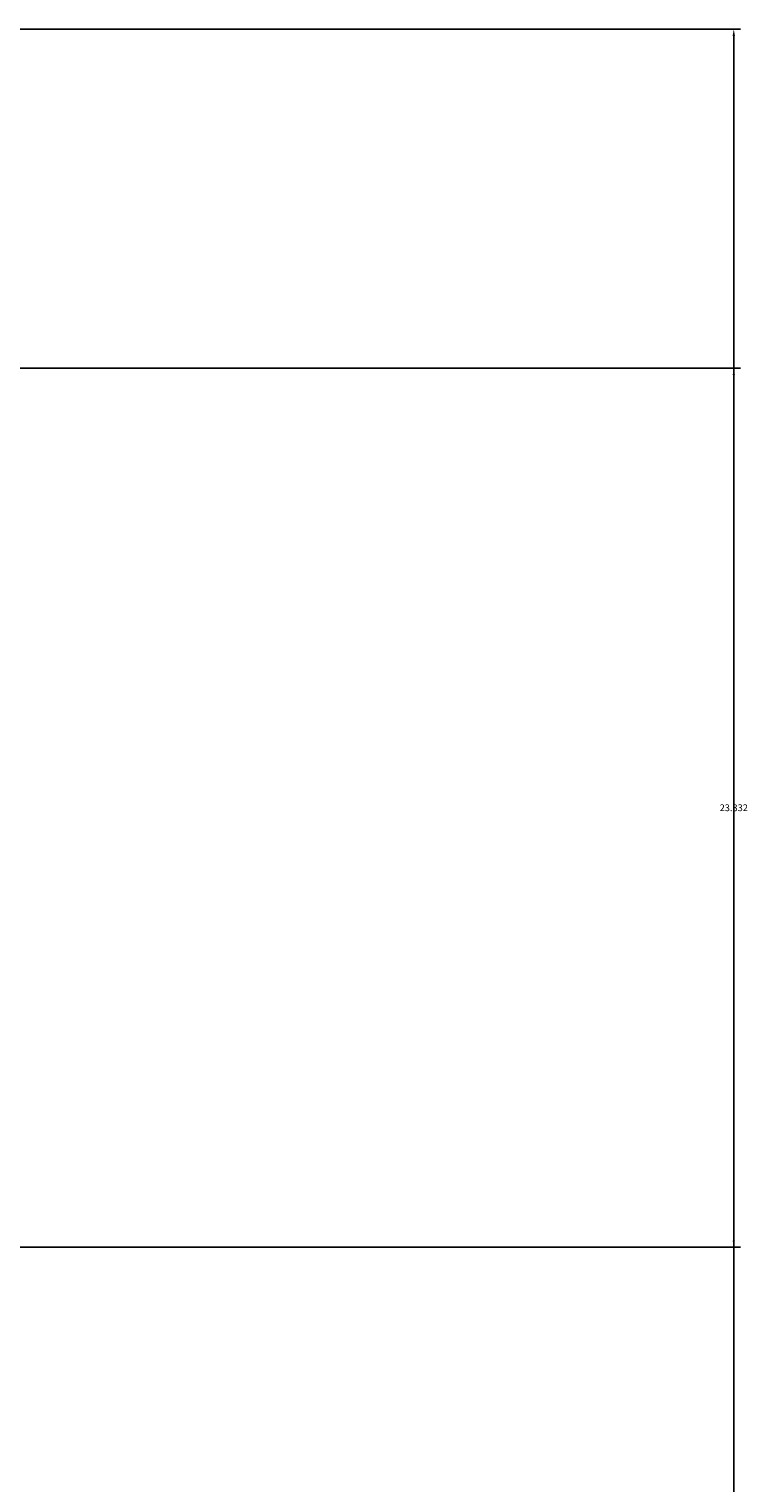
# Model space of a CAD drawing. Units: inches. Extents: x 2307 to 2544, y 2171 to 2540.
# Tile 51 of 52: x 2525 to 2544, y 2482 to 2521. Entities that reach past the tile are written whole.
import ezdxf

# ---------------------------------------------------------------- set-up
doc = ezdxf.new("R2010")
doc.units = ezdxf.units.IN
doc.layers.add('A-ANNO-DIMS', color=2, linetype='Continuous', lineweight=18)
doc.styles.get("Standard").update_dxf_attribs({"font": 'arial.ttf'})
doc.dimstyles.get("Standard").update_dxf_attribs({"dimtxt": 0.18, "dimasz": 0.18, "dimexe": 0.18, "dimexo": 0.0625, "dimgap": 0.09, "dimtad": 0, "dimtih": 1, "dimtoh": 1, "dimdec": 4, "dimzin": 0, "dimdsep": 46, "dimtxsty": 'Standard', "dimcen": 0.09, "dimadec": 0, "dimazin": 0, "dimtfac": 1, "dimtdec": 4, "dimtofl": 0, "dimtmove": 0, "dimatfit": 3, "dimfxl": 1, "dimtolj": 1, "dimtzin": 0, "dimarcsym": 0})

# ---------------------------------------------------------------- blocks, each defined once
blk = doc.blocks.new('*D37')
at = {"layer": 'A-ANNO-DIMS', "color": 0, "lineweight": -2, "transparency": 16777216}
for p, q in [((2524.758, 2520.51), (2544.026, 2520.51)), ((2543.846, 2520.33), (2543.846, 2355.692)), ((2543.846, 2190.69), (2543.846, 2355.328)), ((2524.758, 2190.51), (2544.026, 2190.51))]:
    blk.add_line(p, q, dxfattribs=at)
at = {"layer": 'A-ANNO-DIMS', "color": 0, "transparency": 16777216}
for points in [[(2543.816, 2520.33), (2543.876, 2520.33), (2543.846, 2520.51)], [(2543.816, 2190.69), (2543.876, 2190.69), (2543.846, 2190.51)]]:
    blk.add_solid(points, dxfattribs=at)
at = {"layer": 'Defpoints', "color": 0, "transparency": 16777216}
for p in [(2524.696, 2520.51), (2543.846, 2520.51), (2524.696, 2190.51)]:
    blk.add_point(p, dxfattribs=at)
at = {"layer": 'A-ANNO-DIMS', "color": 0, "transparency": 16777216, "insert": (2543.846, 2355.51), "char_height": 0.18, "attachment_point": 5}
blk.add_mtext('\\A1;330', dxfattribs=at)
blk = doc.blocks.new('*D64')
at = {"layer": 'A-ANNO-DIMS', "color": 0, "lineweight": -2, "transparency": 16777216}
for p, q in [((2515.758, 2511.51), (2544.026, 2511.51)), ((2543.846, 2511.33), (2543.846, 2500.025)), ((2543.846, 2488.357), (2543.846, 2499.661)), ((2514.64, 2488.177), (2544.026, 2488.177))]:
    blk.add_line(p, q, dxfattribs=at)
at = {"layer": 'A-ANNO-DIMS', "color": 0, "transparency": 16777216}
for points in [[(2543.816, 2511.33), (2543.876, 2511.33), (2543.846, 2511.51)], [(2543.816, 2488.357), (2543.876, 2488.357), (2543.846, 2488.177)]]:
    blk.add_solid(points, dxfattribs=at)
at = {"layer": 'Defpoints', "color": 0, "transparency": 16777216}
for p in [(2515.696, 2511.51), (2514.578, 2488.177), (2543.846, 2488.177)]:
    blk.add_point(p, dxfattribs=at)
at = {"layer": 'A-ANNO-DIMS', "color": 0, "transparency": 16777216, "insert": (2543.846, 2499.843), "char_height": 0.18, "attachment_point": 5}
blk.add_mtext('\\A1;23.332', dxfattribs=at)

msp = doc.modelspace()

# ---------------------------------------------------------------- dimensions: what is measured, and where the dimension line sits
at = {"layer": 'A-ANNO-DIMS'}
for base, p1, p2, override, picture, middle in [((2543.8458, 2520.5096), (2524.6958, 2190.5096), (2524.6958, 2520.5096), {"dimdec": 0, "dimlfac": 1, "dimrnd": 0, "dimzin": 0, "dimdsep": 46, "dimlunit": 2}, '*D37', (2543.8458, 2355.5096)), ((2543.8458, 2488.1772), (2515.6958, 2511.5096), (2514.5778, 2488.1772), {"dimdec": 3, "dimlfac": 1, "dimrnd": 0, "dimzin": 0, "dimdsep": 46, "dimlunit": 2}, '*D64', (2543.8458, 2499.8434))]:
    dim = msp.add_linear_dim(base=base, p1=p1, p2=p2, angle=90, dimstyle='Standard', override=override, dxfattribs=at)
    dim.commit()
    dim.dimension.update_dxf_attribs({"geometry": picture, "text_midpoint": middle})

doc.saveas('drawing.dxf')
